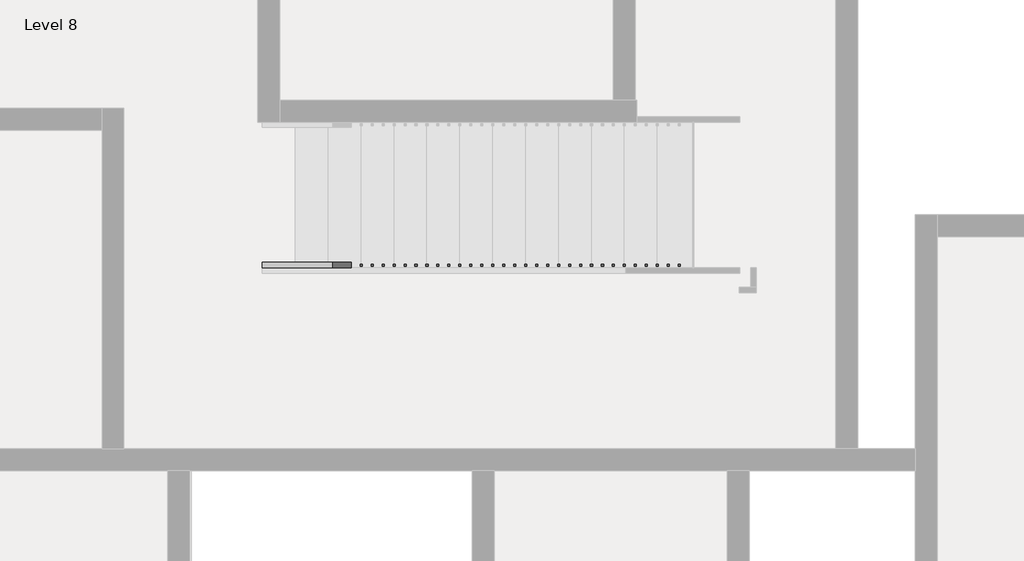
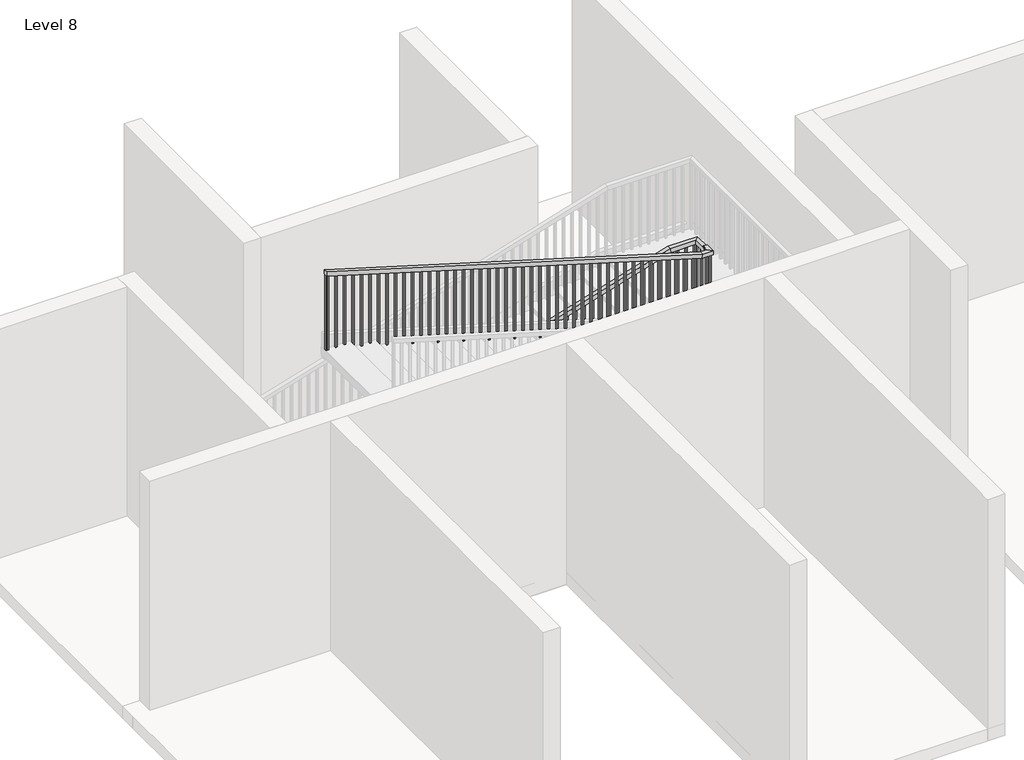
# One storey, part 11 of 14: 1 railing.
"""IFC4 building model written with IfcOpenShell, lengths in millimetres."""

from ifc_helpers import new_model, si_unit, frame, origin, place, context, project, spatial, polyline, outline, extrude, faceted_brep, element, save

model = new_model("IFC4")

# Units and contexts
model_context = context("Model", 3, world=origin())
ifc_project = project(units=[si_unit("LENGTHUNIT", "METRE", prefix="MILLI")], contexts=[model_context])

# Site, building, storey
site = spatial("IfcSite", under=ifc_project)
building = spatial("IfcBuilding", under=site)
storey = spatial("IfcBuildingStorey", under=building, Name="Level 8", Elevation=21336.0)

# Railing
placement = place(None, origin())
element("IfcRailing", 1, ObjectType="Handrail - Rectangular", at=placement, inside=storey, context=model_context, shape_type="SolidModel", body=[
    faceted_brep([(-5254.0891351, 11205.0082924, 22341.84), (-5254.0891351, 11205.0082924, 22288.8032429), (-5254.0891351, 11154.2082924, 22288.8032429), (-5254.0891351, 11154.2082924, 22341.84), (-986.8891351, 11205.0082924, 23622.0), (-979.4332782, 11205.0082924, 23571.2), (-979.4332782, 11154.2082924, 23571.2), (-986.8891351, 11154.2082924, 23622.0), (-631.2891351, 11205.0082924, 23622.0), (-631.2891351, 11205.0082924, 23571.2), (-682.0891351, 11154.2082924, 23571.2), (-682.0891351, 11154.2082924, 23622.0), (-631.2891351, 11001.8082924, 23622.0), (-631.2891351, 10951.0082924, 23571.2), (-682.0891351, 10951.0082924, 23571.2), (-682.0891351, 11001.8082924, 23622.0), (-631.2891351, 11001.8082924, 23644.86), (-631.2891351, 10951.0082924, 23594.06), (-682.0891351, 10951.0082924, 23594.06), (-682.0891351, 11001.8082924, 23644.86), (-631.2891351, 10874.8082924, 23644.86), (-631.2891351, 10874.8082924, 23594.06), (-682.0891351, 10925.6082924, 23594.06), (-682.0891351, 10925.6082924, 23644.86), (-758.2891351, 10874.8082924, 23644.86), (-765.744992, 10874.8082924, 23594.06), (-765.744992, 10925.6082924, 23594.06), (-758.2891351, 10925.6082924, 23644.86), (-5254.0891351, 10874.8082924, 24993.6), (-5254.0891351, 10925.6082924, 24993.6), (-5254.0891351, 10925.6082924, 24940.5632429), (-5254.0891351, 10874.8082924, 24940.5632429)], [[[0, 1, 2, 3]], [[1, 0, 4, 5]], [[2, 1, 5, 6]], [[3, 2, 6, 7]], [[0, 3, 7, 4]], [[5, 4, 8, 9]], [[6, 5, 9, 10]], [[7, 6, 10, 11]], [[4, 7, 11, 8]], [[9, 8, 12, 13]], [[10, 9, 13, 14]], [[11, 10, 14, 15]], [[8, 11, 15, 12]], [[13, 12, 16, 17]], [[14, 13, 17, 18]], [[15, 14, 18, 19]], [[12, 15, 19, 16]], [[17, 16, 20, 21]], [[18, 17, 21, 22]], [[19, 18, 22, 23]], [[16, 19, 23, 20]], [[21, 20, 24, 25]], [[22, 21, 25, 26]], [[23, 22, 26, 27]], [[20, 23, 27, 24]], [[28, 29, 30, 31]], [[25, 24, 28, 31]], [[26, 25, 31, 30]], [[27, 26, 30, 29]], [[24, 27, 29, 28]]]),
    extrude(outline(polyline([(24930.0857429, -5219.1641351), (24935.8007429, -5238.2141351), (23987.76, -5238.2141351), (23987.76, -5219.1641351), (24930.0857429, -5219.1641351)])), frame((0.0, 10890.6832924, 0.0), z_axis=(0.0, 1.0, 0.0), x_axis=(0.0, 0.0, 1.0)), (0.0, 0.0, 1.0), 19.05),
    extrude(outline(polyline([(24899.6057429, -5117.5641351), (24905.3207429, -5136.6141351), (23987.76, -5136.6141351), (23987.76, -5117.5641351), (24899.6057429, -5117.5641351)])), frame((0.0, 10890.6832924, 0.0), z_axis=(0.0, 1.0, 0.0), x_axis=(0.0, 0.0, 1.0)), (0.0, 0.0, 1.0), 19.05),
    extrude(outline(polyline([(24869.1257429, -5015.9641351), (24874.8407429, -5035.0141351), (23987.76, -5035.0141351), (23987.76, -5015.9641351), (24869.1257429, -5015.9641351)])), frame((0.0, 10890.6832924, 0.0), z_axis=(0.0, 1.0, 0.0), x_axis=(0.0, 0.0, 1.0)), (0.0, 0.0, 1.0), 19.05),
    extrude(outline(polyline([(24838.6457429, -4914.3641351), (24844.3607429, -4933.4141351), (23896.32, -4933.4141351), (23896.32, -4914.3641351), (24838.6457429, -4914.3641351)])), frame((0.0, 10890.6832924, 0.0), z_axis=(0.0, 1.0, 0.0), x_axis=(0.0, 0.0, 1.0)), (0.0, 0.0, 1.0), 19.05),
    extrude(outline(polyline([(24808.1657429, -4812.7641351), (24813.8807429, -4831.8141351), (23896.32, -4831.8141351), (23896.32, -4812.7641351), (24808.1657429, -4812.7641351)])), frame((0.0, 10890.6832924, 0.0), z_axis=(0.0, 1.0, 0.0), x_axis=(0.0, 0.0, 1.0)), (0.0, 0.0, 1.0), 19.05),
    extrude(outline(polyline([(24777.6857429, -4711.1641351), (24783.4007429, -4730.2141351), (23896.32, -4730.2141351), (23896.32, -4711.1641351), (24777.6857429, -4711.1641351)])), frame((0.0, 10890.6832924, 0.0), z_axis=(0.0, 1.0, 0.0), x_axis=(0.0, 0.0, 1.0)), (0.0, 0.0, 1.0), 19.05),
    extrude(outline(polyline([(24747.2057429, -4609.5641351), (24752.9207429, -4628.6141351), (23804.88, -4628.6141351), (23804.88, -4609.5641351), (24747.2057429, -4609.5641351)])), frame((0.0, 10890.6832924, 0.0), z_axis=(0.0, 1.0, 0.0), x_axis=(0.0, 0.0, 1.0)), (0.0, 0.0, 1.0), 19.05),
    extrude(outline(polyline([(24716.7257429, -4507.9641351), (24722.4407429, -4527.0141351), (23804.88, -4527.0141351), (23804.88, -4507.9641351), (24716.7257429, -4507.9641351)])), frame((0.0, 10890.6832924, 0.0), z_axis=(0.0, 1.0, 0.0), x_axis=(0.0, 0.0, 1.0)), (0.0, 0.0, 1.0), 19.05),
    extrude(outline(polyline([(24686.2457429, -4406.3641351), (24691.9607429, -4425.4141351), (23804.88, -4425.4141351), (23804.88, -4406.3641351), (24686.2457429, -4406.3641351)])), frame((0.0, 10890.6832924, 0.0), z_axis=(0.0, 1.0, 0.0), x_axis=(0.0, 0.0, 1.0)), (0.0, 0.0, 1.0), 19.05),
    extrude(outline(polyline([(24655.7657429, -4304.7641351), (24661.4807429, -4323.8141351), (23713.44, -4323.8141351), (23713.44, -4304.7641351), (24655.7657429, -4304.7641351)])), frame((0.0, 10890.6832924, 0.0), z_axis=(0.0, 1.0, 0.0), x_axis=(0.0, 0.0, 1.0)), (0.0, 0.0, 1.0), 19.05),
    extrude(outline(polyline([(24625.2857429, -4203.1641351), (24631.0007429, -4222.2141351), (23713.44, -4222.2141351), (23713.44, -4203.1641351), (24625.2857429, -4203.1641351)])), frame((0.0, 10890.6832924, 0.0), z_axis=(0.0, 1.0, 0.0), x_axis=(0.0, 0.0, 1.0)), (0.0, 0.0, 1.0), 19.05),
    extrude(outline(polyline([(24594.8057429, -4101.5641351), (24600.5207429, -4120.6141351), (23713.44, -4120.6141351), (23713.44, -4101.5641351), (24594.8057429, -4101.5641351)])), frame((0.0, 10890.6832924, 0.0), z_axis=(0.0, 1.0, 0.0), x_axis=(0.0, 0.0, 1.0)), (0.0, 0.0, 1.0), 19.05),
    extrude(outline(polyline([(24564.3257429, -3999.9641351), (24570.0407429, -4019.0141351), (23622.0, -4019.0141351), (23622.0, -3999.9641351), (24564.3257429, -3999.9641351)])), frame((0.0, 10890.6832924, 0.0), z_axis=(0.0, 1.0, 0.0), x_axis=(0.0, 0.0, 1.0)), (0.0, 0.0, 1.0), 19.05),
    extrude(outline(polyline([(24533.8457429, -3898.3641351), (24539.5607429, -3917.4141351), (23622.0, -3917.4141351), (23622.0, -3898.3641351), (24533.8457429, -3898.3641351)])), frame((0.0, 10890.6832924, 0.0), z_axis=(0.0, 1.0, 0.0), x_axis=(0.0, 0.0, 1.0)), (0.0, 0.0, 1.0), 19.05),
    extrude(outline(polyline([(24503.3657429, -3796.7641351), (24509.0807429, -3815.8141351), (23622.0, -3815.8141351), (23622.0, -3796.7641351), (24503.3657429, -3796.7641351)])), frame((0.0, 10890.6832924, 0.0), z_axis=(0.0, 1.0, 0.0), x_axis=(0.0, 0.0, 1.0)), (0.0, 0.0, 1.0), 19.05),
    extrude(outline(polyline([(24472.8857429, -3695.1641351), (24478.6007429, -3714.2141351), (23530.56, -3714.2141351), (23530.56, -3695.1641351), (24472.8857429, -3695.1641351)])), frame((0.0, 10890.6832924, 0.0), z_axis=(0.0, 1.0, 0.0), x_axis=(0.0, 0.0, 1.0)), (0.0, 0.0, 1.0), 19.05),
    extrude(outline(polyline([(24442.4057429, -3593.5641351), (24448.1207429, -3612.6141351), (23530.56, -3612.6141351), (23530.56, -3593.5641351), (24442.4057429, -3593.5641351)])), frame((0.0, 10890.6832924, 0.0), z_axis=(0.0, 1.0, 0.0), x_axis=(0.0, 0.0, 1.0)), (0.0, 0.0, 1.0), 19.05),
    extrude(outline(polyline([(24411.9257429, -3491.9641351), (24417.6407429, -3511.0141351), (23530.56, -3511.0141351), (23530.56, -3491.9641351), (24411.9257429, -3491.9641351)])), frame((0.0, 10890.6832924, 0.0), z_axis=(0.0, 1.0, 0.0), x_axis=(0.0, 0.0, 1.0)), (0.0, 0.0, 1.0), 19.05),
    extrude(outline(polyline([(24381.4457429, -3390.3641351), (24387.1607429, -3409.4141351), (23439.12, -3409.4141351), (23439.12, -3390.3641351), (24381.4457429, -3390.3641351)])), frame((0.0, 10890.6832924, 0.0), z_axis=(0.0, 1.0, 0.0), x_axis=(0.0, 0.0, 1.0)), (0.0, 0.0, 1.0), 19.05),
    extrude(outline(polyline([(24350.9657429, -3288.7641351), (24356.6807429, -3307.8141351), (23439.12, -3307.8141351), (23439.12, -3288.7641351), (24350.9657429, -3288.7641351)])), frame((0.0, 10890.6832924, 0.0), z_axis=(0.0, 1.0, 0.0), x_axis=(0.0, 0.0, 1.0)), (0.0, 0.0, 1.0), 19.05),
    extrude(outline(polyline([(24320.4857429, -3187.1641351), (24326.2007429, -3206.2141351), (23439.12, -3206.2141351), (23439.12, -3187.1641351), (24320.4857429, -3187.1641351)])), frame((0.0, 10890.6832924, 0.0), z_axis=(0.0, 1.0, 0.0), x_axis=(0.0, 0.0, 1.0)), (0.0, 0.0, 1.0), 19.05),
    extrude(outline(polyline([(24290.0057429, -3085.5641351), (24295.7207429, -3104.6141351), (23347.68, -3104.6141351), (23347.68, -3085.5641351), (24290.0057429, -3085.5641351)])), frame((0.0, 10890.6832924, 0.0), z_axis=(0.0, 1.0, 0.0), x_axis=(0.0, 0.0, 1.0)), (0.0, 0.0, 1.0), 19.05),
    extrude(outline(polyline([(24259.5257429, -2983.9641351), (24265.2407429, -3003.0141351), (23347.68, -3003.0141351), (23347.68, -2983.9641351), (24259.5257429, -2983.9641351)])), frame((0.0, 10890.6832924, 0.0), z_axis=(0.0, 1.0, 0.0), x_axis=(0.0, 0.0, 1.0)), (0.0, 0.0, 1.0), 19.05),
    extrude(outline(polyline([(24229.0457429, -2882.3641351), (24234.7607429, -2901.4141351), (23347.68, -2901.4141351), (23347.68, -2882.3641351), (24229.0457429, -2882.3641351)])), frame((0.0, 10890.6832924, 0.0), z_axis=(0.0, 1.0, 0.0), x_axis=(0.0, 0.0, 1.0)), (0.0, 0.0, 1.0), 19.05),
    extrude(outline(polyline([(24198.5657429, -2780.7641351), (24204.2807429, -2799.8141351), (23256.24, -2799.8141351), (23256.24, -2780.7641351), (24198.5657429, -2780.7641351)])), frame((0.0, 10890.6832924, 0.0), z_axis=(0.0, 1.0, 0.0), x_axis=(0.0, 0.0, 1.0)), (0.0, 0.0, 1.0), 19.05),
    extrude(outline(polyline([(24168.0857429, -2679.1641351), (24173.8007429, -2698.2141351), (23256.24, -2698.2141351), (23256.24, -2679.1641351), (24168.0857429, -2679.1641351)])), frame((0.0, 10890.6832924, 0.0), z_axis=(0.0, 1.0, 0.0), x_axis=(0.0, 0.0, 1.0)), (0.0, 0.0, 1.0), 19.05),
    extrude(outline(polyline([(24137.6057429, -2577.5641351), (24143.3207429, -2596.6141351), (23256.24, -2596.6141351), (23256.24, -2577.5641351), (24137.6057429, -2577.5641351)])), frame((0.0, 10890.6832924, 0.0), z_axis=(0.0, 1.0, 0.0), x_axis=(0.0, 0.0, 1.0)), (0.0, 0.0, 1.0), 19.05),
    extrude(outline(polyline([(24107.1257429, -2475.9641351), (24112.8407429, -2495.0141351), (23164.8, -2495.0141351), (23164.8, -2475.9641351), (24107.1257429, -2475.9641351)])), frame((0.0, 10890.6832924, 0.0), z_axis=(0.0, 1.0, 0.0), x_axis=(0.0, 0.0, 1.0)), (0.0, 0.0, 1.0), 19.05),
    extrude(outline(polyline([(24076.6457429, -2374.3641351), (24082.3607429, -2393.4141351), (23164.8, -2393.4141351), (23164.8, -2374.3641351), (24076.6457429, -2374.3641351)])), frame((0.0, 10890.6832924, 0.0), z_axis=(0.0, 1.0, 0.0), x_axis=(0.0, 0.0, 1.0)), (0.0, 0.0, 1.0), 19.05),
    extrude(outline(polyline([(24046.1657429, -2272.7641351), (24051.8807429, -2291.8141351), (23164.8, -2291.8141351), (23164.8, -2272.7641351), (24046.1657429, -2272.7641351)])), frame((0.0, 10890.6832924, 0.0), z_axis=(0.0, 1.0, 0.0), x_axis=(0.0, 0.0, 1.0)), (0.0, 0.0, 1.0), 19.05),
    extrude(outline(polyline([(24015.6857429, -2171.1641351), (24021.4007429, -2190.2141351), (23073.36, -2190.2141351), (23073.36, -2171.1641351), (24015.6857429, -2171.1641351)])), frame((0.0, 10890.6832924, 0.0), z_axis=(0.0, 1.0, 0.0), x_axis=(0.0, 0.0, 1.0)), (0.0, 0.0, 1.0), 19.05),
    extrude(outline(polyline([(23985.2057429, -2069.5641351), (23990.9207429, -2088.6141351), (23073.36, -2088.6141351), (23073.36, -2069.5641351), (23985.2057429, -2069.5641351)])), frame((0.0, 10890.6832924, 0.0), z_axis=(0.0, 1.0, 0.0), x_axis=(0.0, 0.0, 1.0)), (0.0, 0.0, 1.0), 19.05),
    extrude(outline(polyline([(23954.7257429, -1967.9641351), (23960.4407429, -1987.0141351), (23073.36, -1987.0141351), (23073.36, -1967.9641351), (23954.7257429, -1967.9641351)])), frame((0.0, 10890.6832924, 0.0), z_axis=(0.0, 1.0, 0.0), x_axis=(0.0, 0.0, 1.0)), (0.0, 0.0, 1.0), 19.05),
    extrude(outline(polyline([(23924.2457429, -1866.3641351), (23929.9607429, -1885.4141351), (22981.92, -1885.4141351), (22981.92, -1866.3641351), (23924.2457429, -1866.3641351)])), frame((0.0, 10890.6832924, 0.0), z_axis=(0.0, 1.0, 0.0), x_axis=(0.0, 0.0, 1.0)), (0.0, 0.0, 1.0), 19.05),
    extrude(outline(polyline([(23893.7657429, -1764.7641351), (23899.4807429, -1783.8141351), (22981.92, -1783.8141351), (22981.92, -1764.7641351), (23893.7657429, -1764.7641351)])), frame((0.0, 10890.6832924, 0.0), z_axis=(0.0, 1.0, 0.0), x_axis=(0.0, 0.0, 1.0)), (0.0, 0.0, 1.0), 19.05),
    extrude(outline(polyline([(23863.2857429, -1663.1641351), (23869.0007429, -1682.2141351), (22981.92, -1682.2141351), (22981.92, -1663.1641351), (23863.2857429, -1663.1641351)])), frame((0.0, 10890.6832924, 0.0), z_axis=(0.0, 1.0, 0.0), x_axis=(0.0, 0.0, 1.0)), (0.0, 0.0, 1.0), 19.05),
    extrude(outline(polyline([(23832.8057429, -1561.5641351), (23838.5207429, -1580.6141351), (22890.48, -1580.6141351), (22890.48, -1561.5641351), (23832.8057429, -1561.5641351)])), frame((0.0, 10890.6832924, 0.0), z_axis=(0.0, 1.0, 0.0), x_axis=(0.0, 0.0, 1.0)), (0.0, 0.0, 1.0), 19.05),
    extrude(outline(polyline([(23802.3257429, -1459.9641351), (23808.0407429, -1479.0141351), (22890.48, -1479.0141351), (22890.48, -1459.9641351), (23802.3257429, -1459.9641351)])), frame((0.0, 10890.6832924, 0.0), z_axis=(0.0, 1.0, 0.0), x_axis=(0.0, 0.0, 1.0)), (0.0, 0.0, 1.0), 19.05),
    extrude(outline(polyline([(23771.8457429, -1358.3641351), (23777.5607429, -1377.4141351), (22890.48, -1377.4141351), (22890.48, -1358.3641351), (23771.8457429, -1358.3641351)])), frame((0.0, 10890.6832924, 0.0), z_axis=(0.0, 1.0, 0.0), x_axis=(0.0, 0.0, 1.0)), (0.0, 0.0, 1.0), 19.05),
    extrude(outline(polyline([(23741.3657429, -1256.7641351), (23747.0807429, -1275.8141351), (22799.04, -1275.8141351), (22799.04, -1256.7641351), (23741.3657429, -1256.7641351)])), frame((0.0, 10890.6832924, 0.0), z_axis=(0.0, 1.0, 0.0), x_axis=(0.0, 0.0, 1.0)), (0.0, 0.0, 1.0), 19.05),
    extrude(outline(polyline([(23710.8857429, -1155.1641351), (23716.6007429, -1174.2141351), (22799.04, -1174.2141351), (22799.04, -1155.1641351), (23710.8857429, -1155.1641351)])), frame((0.0, 10890.6832924, 0.0), z_axis=(0.0, 1.0, 0.0), x_axis=(0.0, 0.0, 1.0)), (0.0, 0.0, 1.0), 19.05),
    extrude(outline(polyline([(23680.4057429, -1053.5641351), (23686.1207429, -1072.6141351), (22799.04, -1072.6141351), (22799.04, -1053.5641351), (23680.4057429, -1053.5641351)])), frame((0.0, 10890.6832924, 0.0), z_axis=(0.0, 1.0, 0.0), x_axis=(0.0, 0.0, 1.0)), (0.0, 0.0, 1.0), 19.05),
    extrude(outline(polyline([(23649.9257429, -951.9641351), (23655.6407429, -971.0141351), (22707.6, -971.0141351), (22707.6, -951.9641351), (23649.9257429, -951.9641351)])), frame((0.0, 10890.6832924, 0.0), z_axis=(0.0, 1.0, 0.0), x_axis=(0.0, 0.0, 1.0)), (0.0, 0.0, 1.0), 19.05),
    extrude(outline(polyline([(23619.4457429, -850.3641351), (23625.1607429, -869.4141351), (22707.6, -869.4141351), (22707.6, -850.3641351), (23619.4457429, -850.3641351)])), frame((0.0, 10890.6832924, 0.0), z_axis=(0.0, 1.0, 0.0), x_axis=(0.0, 0.0, 1.0)), (0.0, 0.0, 1.0), 19.05),
    extrude(outline(polyline([(23588.9657429, -748.7641351), (23594.6807429, -767.8141351), (22707.6, -767.8141351), (22707.6, -748.7641351), (23588.9657429, -748.7641351)])), frame((0.0, 10890.6832924, 0.0), z_axis=(0.0, 1.0, 0.0), x_axis=(0.0, 0.0, 1.0)), (0.0, 0.0, 1.0), 19.05),
    extrude(outline(polyline([(-666.2141351, 10985.9332924), (-647.1641351, 10985.9332924), (-647.1641351, 10966.8832924), (-666.2141351, 10966.8832924), (-666.2141351, 10985.9332924)])), frame((0.0, 0.0, 22707.6), z_axis=(0.0, 0.0, 1.0), x_axis=(1.0, 0.0, 0.0)), (0.0, 0.0, 1.0), 886.46),
    extrude(outline(polyline([(-666.2141351, 11087.5332924), (-647.1641351, 11087.5332924), (-647.1641351, 11068.4832924), (-666.2141351, 11068.4832924), (-666.2141351, 11087.5332924)])), frame((0.0, 0.0, 22707.6), z_axis=(0.0, 0.0, 1.0), x_axis=(1.0, 0.0, 0.0)), (0.0, 0.0, 1.0), 863.6),
    extrude(outline(polyline([(-691.6141351, 11170.0832924), (-691.6141351, 11189.1332924), (-672.5641351, 11189.1332924), (-672.5641351, 11170.0832924), (-691.6141351, 11170.0832924)])), frame((0.0, 0.0, 22707.6), z_axis=(0.0, 0.0, 1.0), x_axis=(1.0, 0.0, 0.0)), (0.0, 0.0, 1.0), 863.6),
    extrude(outline(polyline([(-793.2141351, 11170.0832924), (-793.2141351, 11189.1332924), (-774.1641351, 11189.1332924), (-774.1641351, 11170.0832924), (-793.2141351, 11170.0832924)])), frame((0.0, 0.0, 22707.6), z_axis=(0.0, 0.0, 1.0), x_axis=(1.0, 0.0, 0.0)), (0.0, 0.0, 1.0), 863.6),
    extrude(outline(polyline([(-894.8141351, 11170.0832924), (-894.8141351, 11189.1332924), (-875.7641351, 11189.1332924), (-875.7641351, 11170.0832924), (-894.8141351, 11170.0832924)])), frame((0.0, 0.0, 22707.6), z_axis=(0.0, 0.0, 1.0), x_axis=(1.0, 0.0, 0.0)), (0.0, 0.0, 1.0), 863.6),
    extrude(outline(polyline([(23571.8207429, -977.3641351), (23566.1057429, -996.4141351), (22707.6, -996.4141351), (22707.6, -977.3641351), (23571.8207429, -977.3641351)])), frame((0.0, 11170.0832924, 0.0), z_axis=(0.0, 1.0, 0.0), x_axis=(0.0, 0.0, 1.0)), (0.0, 0.0, 1.0), 19.05),
    extrude(outline(polyline([(23541.3407429, -1078.9641351), (23535.6257429, -1098.0141351), (22616.16, -1098.0141351), (22616.16, -1078.9641351), (23541.3407429, -1078.9641351)])), frame((0.0, 11170.0832924, 0.0), z_axis=(0.0, 1.0, 0.0), x_axis=(0.0, 0.0, 1.0)), (0.0, 0.0, 1.0), 19.05),
    extrude(outline(polyline([(23510.8607429, -1180.5641351), (23505.1457429, -1199.6141351), (22616.16, -1199.6141351), (22616.16, -1180.5641351), (23510.8607429, -1180.5641351)])), frame((0.0, 11170.0832924, 0.0), z_axis=(0.0, 1.0, 0.0), x_axis=(0.0, 0.0, 1.0)), (0.0, 0.0, 1.0), 19.05),
    extrude(outline(polyline([(23480.3807429, -1282.1641351), (23474.6657429, -1301.2141351), (22616.16, -1301.2141351), (22616.16, -1282.1641351), (23480.3807429, -1282.1641351)])), frame((0.0, 11170.0832924, 0.0), z_axis=(0.0, 1.0, 0.0), x_axis=(0.0, 0.0, 1.0)), (0.0, 0.0, 1.0), 19.05),
    extrude(outline(polyline([(23449.9007429, -1383.7641351), (23444.1857429, -1402.8141351), (22524.72, -1402.8141351), (22524.72, -1383.7641351), (23449.9007429, -1383.7641351)])), frame((0.0, 11170.0832924, 0.0), z_axis=(0.0, 1.0, 0.0), x_axis=(0.0, 0.0, 1.0)), (0.0, 0.0, 1.0), 19.05),
    extrude(outline(polyline([(23419.4207429, -1485.3641351), (23413.7057429, -1504.4141351), (22524.72, -1504.4141351), (22524.72, -1485.3641351), (23419.4207429, -1485.3641351)])), frame((0.0, 11170.0832924, 0.0), z_axis=(0.0, 1.0, 0.0), x_axis=(0.0, 0.0, 1.0)), (0.0, 0.0, 1.0), 19.05),
    extrude(outline(polyline([(23388.9407429, -1586.9641351), (23383.2257429, -1606.0141351), (22524.72, -1606.0141351), (22524.72, -1586.9641351), (23388.9407429, -1586.9641351)])), frame((0.0, 11170.0832924, 0.0), z_axis=(0.0, 1.0, 0.0), x_axis=(0.0, 0.0, 1.0)), (0.0, 0.0, 1.0), 19.05),
    extrude(outline(polyline([(23358.4607429, -1688.5641351), (23352.7457429, -1707.6141351), (22433.28, -1707.6141351), (22433.28, -1688.5641351), (23358.4607429, -1688.5641351)])), frame((0.0, 11170.0832924, 0.0), z_axis=(0.0, 1.0, 0.0), x_axis=(0.0, 0.0, 1.0)), (0.0, 0.0, 1.0), 19.05),
    extrude(outline(polyline([(23327.9807429, -1790.1641351), (23322.2657429, -1809.2141351), (22433.28, -1809.2141351), (22433.28, -1790.1641351), (23327.9807429, -1790.1641351)])), frame((0.0, 11170.0832924, 0.0), z_axis=(0.0, 1.0, 0.0), x_axis=(0.0, 0.0, 1.0)), (0.0, 0.0, 1.0), 19.05),
    extrude(outline(polyline([(23297.5007429, -1891.7641351), (23291.7857429, -1910.8141351), (22433.28, -1910.8141351), (22433.28, -1891.7641351), (23297.5007429, -1891.7641351)])), frame((0.0, 11170.0832924, 0.0), z_axis=(0.0, 1.0, 0.0), x_axis=(0.0, 0.0, 1.0)), (0.0, 0.0, 1.0), 19.05),
    extrude(outline(polyline([(23267.0207429, -1993.3641351), (23261.3057429, -2012.4141351), (22341.84, -2012.4141351), (22341.84, -1993.3641351), (23267.0207429, -1993.3641351)])), frame((0.0, 11170.0832924, 0.0), z_axis=(0.0, 1.0, 0.0), x_axis=(0.0, 0.0, 1.0)), (0.0, 0.0, 1.0), 19.05),
    extrude(outline(polyline([(23236.5407429, -2094.9641351), (23230.8257429, -2114.0141351), (22341.84, -2114.0141351), (22341.84, -2094.9641351), (23236.5407429, -2094.9641351)])), frame((0.0, 11170.0832924, 0.0), z_axis=(0.0, 1.0, 0.0), x_axis=(0.0, 0.0, 1.0)), (0.0, 0.0, 1.0), 19.05),
    extrude(outline(polyline([(23206.0607429, -2196.5641351), (23200.3457429, -2215.6141351), (22341.84, -2215.6141351), (22341.84, -2196.5641351), (23206.0607429, -2196.5641351)])), frame((0.0, 11170.0832924, 0.0), z_axis=(0.0, 1.0, 0.0), x_axis=(0.0, 0.0, 1.0)), (0.0, 0.0, 1.0), 19.05),
    extrude(outline(polyline([(23175.5807429, -2298.1641351), (23169.8657429, -2317.2141351), (22250.4, -2317.2141351), (22250.4, -2298.1641351), (23175.5807429, -2298.1641351)])), frame((0.0, 11170.0832924, 0.0), z_axis=(0.0, 1.0, 0.0), x_axis=(0.0, 0.0, 1.0)), (0.0, 0.0, 1.0), 19.05),
    extrude(outline(polyline([(23145.1007429, -2399.7641351), (23139.3857429, -2418.8141351), (22250.4, -2418.8141351), (22250.4, -2399.7641351), (23145.1007429, -2399.7641351)])), frame((0.0, 11170.0832924, 0.0), z_axis=(0.0, 1.0, 0.0), x_axis=(0.0, 0.0, 1.0)), (0.0, 0.0, 1.0), 19.05),
    extrude(outline(polyline([(23114.6207429, -2501.3641351), (23108.9057429, -2520.4141351), (22250.4, -2520.4141351), (22250.4, -2501.3641351), (23114.6207429, -2501.3641351)])), frame((0.0, 11170.0832924, 0.0), z_axis=(0.0, 1.0, 0.0), x_axis=(0.0, 0.0, 1.0)), (0.0, 0.0, 1.0), 19.05),
    extrude(outline(polyline([(23084.1407429, -2602.9641351), (23078.4257429, -2622.0141351), (22158.96, -2622.0141351), (22158.96, -2602.9641351), (23084.1407429, -2602.9641351)])), frame((0.0, 11170.0832924, 0.0), z_axis=(0.0, 1.0, 0.0), x_axis=(0.0, 0.0, 1.0)), (0.0, 0.0, 1.0), 19.05),
    extrude(outline(polyline([(23053.6607429, -2704.5641351), (23047.9457429, -2723.6141351), (22158.96, -2723.6141351), (22158.96, -2704.5641351), (23053.6607429, -2704.5641351)])), frame((0.0, 11170.0832924, 0.0), z_axis=(0.0, 1.0, 0.0), x_axis=(0.0, 0.0, 1.0)), (0.0, 0.0, 1.0), 19.05),
    extrude(outline(polyline([(23023.1807429, -2806.1641351), (23017.4657429, -2825.2141351), (22158.96, -2825.2141351), (22158.96, -2806.1641351), (23023.1807429, -2806.1641351)])), frame((0.0, 11170.0832924, 0.0), z_axis=(0.0, 1.0, 0.0), x_axis=(0.0, 0.0, 1.0)), (0.0, 0.0, 1.0), 19.05),
    extrude(outline(polyline([(22992.7007429, -2907.7641351), (22986.9857429, -2926.8141351), (22067.52, -2926.8141351), (22067.52, -2907.7641351), (22992.7007429, -2907.7641351)])), frame((0.0, 11170.0832924, 0.0), z_axis=(0.0, 1.0, 0.0), x_axis=(0.0, 0.0, 1.0)), (0.0, 0.0, 1.0), 19.05),
    extrude(outline(polyline([(22962.2207429, -3009.3641351), (22956.5057429, -3028.4141351), (22067.52, -3028.4141351), (22067.52, -3009.3641351), (22962.2207429, -3009.3641351)])), frame((0.0, 11170.0832924, 0.0), z_axis=(0.0, 1.0, 0.0), x_axis=(0.0, 0.0, 1.0)), (0.0, 0.0, 1.0), 19.05),
    extrude(outline(polyline([(22931.7407429, -3110.9641351), (22926.0257429, -3130.0141351), (22067.52, -3130.0141351), (22067.52, -3110.9641351), (22931.7407429, -3110.9641351)])), frame((0.0, 11170.0832924, 0.0), z_axis=(0.0, 1.0, 0.0), x_axis=(0.0, 0.0, 1.0)), (0.0, 0.0, 1.0), 19.05),
    extrude(outline(polyline([(22901.2607429, -3212.5641351), (22895.5457429, -3231.6141351), (21976.08, -3231.6141351), (21976.08, -3212.5641351), (22901.2607429, -3212.5641351)])), frame((0.0, 11170.0832924, 0.0), z_axis=(0.0, 1.0, 0.0), x_axis=(0.0, 0.0, 1.0)), (0.0, 0.0, 1.0), 19.05),
    extrude(outline(polyline([(22870.7807429, -3314.1641351), (22865.0657429, -3333.2141351), (21976.08, -3333.2141351), (21976.08, -3314.1641351), (22870.7807429, -3314.1641351)])), frame((0.0, 11170.0832924, 0.0), z_axis=(0.0, 1.0, 0.0), x_axis=(0.0, 0.0, 1.0)), (0.0, 0.0, 1.0), 19.05),
    extrude(outline(polyline([(22840.3007429, -3415.7641351), (22834.5857429, -3434.8141351), (21976.08, -3434.8141351), (21976.08, -3415.7641351), (22840.3007429, -3415.7641351)])), frame((0.0, 11170.0832924, 0.0), z_axis=(0.0, 1.0, 0.0), x_axis=(0.0, 0.0, 1.0)), (0.0, 0.0, 1.0), 19.05),
    extrude(outline(polyline([(22809.8207429, -3517.3641351), (22804.1057429, -3536.4141351), (21884.64, -3536.4141351), (21884.64, -3517.3641351), (22809.8207429, -3517.3641351)])), frame((0.0, 11170.0832924, 0.0), z_axis=(0.0, 1.0, 0.0), x_axis=(0.0, 0.0, 1.0)), (0.0, 0.0, 1.0), 19.05),
    extrude(outline(polyline([(22779.3407429, -3618.9641351), (22773.6257429, -3638.0141351), (21884.64, -3638.0141351), (21884.64, -3618.9641351), (22779.3407429, -3618.9641351)])), frame((0.0, 11170.0832924, 0.0), z_axis=(0.0, 1.0, 0.0), x_axis=(0.0, 0.0, 1.0)), (0.0, 0.0, 1.0), 19.05),
    extrude(outline(polyline([(22748.8607429, -3720.5641351), (22743.1457429, -3739.6141351), (21884.64, -3739.6141351), (21884.64, -3720.5641351), (22748.8607429, -3720.5641351)])), frame((0.0, 11170.0832924, 0.0), z_axis=(0.0, 1.0, 0.0), x_axis=(0.0, 0.0, 1.0)), (0.0, 0.0, 1.0), 19.05),
    extrude(outline(polyline([(22718.3807429, -3822.1641351), (22712.6657429, -3841.2141351), (21793.2, -3841.2141351), (21793.2, -3822.1641351), (22718.3807429, -3822.1641351)])), frame((0.0, 11170.0832924, 0.0), z_axis=(0.0, 1.0, 0.0), x_axis=(0.0, 0.0, 1.0)), (0.0, 0.0, 1.0), 19.05),
    extrude(outline(polyline([(22687.9007429, -3923.7641351), (22682.1857429, -3942.8141351), (21793.2, -3942.8141351), (21793.2, -3923.7641351), (22687.9007429, -3923.7641351)])), frame((0.0, 11170.0832924, 0.0), z_axis=(0.0, 1.0, 0.0), x_axis=(0.0, 0.0, 1.0)), (0.0, 0.0, 1.0), 19.05),
    extrude(outline(polyline([(22657.4207429, -4025.3641351), (22651.7057429, -4044.4141351), (21793.2, -4044.4141351), (21793.2, -4025.3641351), (22657.4207429, -4025.3641351)])), frame((0.0, 11170.0832924, 0.0), z_axis=(0.0, 1.0, 0.0), x_axis=(0.0, 0.0, 1.0)), (0.0, 0.0, 1.0), 19.05),
    extrude(outline(polyline([(22626.9407429, -4126.9641351), (22621.2257429, -4146.0141351), (21701.76, -4146.0141351), (21701.76, -4126.9641351), (22626.9407429, -4126.9641351)])), frame((0.0, 11170.0832924, 0.0), z_axis=(0.0, 1.0, 0.0), x_axis=(0.0, 0.0, 1.0)), (0.0, 0.0, 1.0), 19.05),
    extrude(outline(polyline([(22596.4607429, -4228.5641351), (22590.7457429, -4247.6141351), (21701.76, -4247.6141351), (21701.76, -4228.5641351), (22596.4607429, -4228.5641351)])), frame((0.0, 11170.0832924, 0.0), z_axis=(0.0, 1.0, 0.0), x_axis=(0.0, 0.0, 1.0)), (0.0, 0.0, 1.0), 19.05),
    extrude(outline(polyline([(22565.9807429, -4330.1641351), (22560.2657429, -4349.2141351), (21701.76, -4349.2141351), (21701.76, -4330.1641351), (22565.9807429, -4330.1641351)])), frame((0.0, 11170.0832924, 0.0), z_axis=(0.0, 1.0, 0.0), x_axis=(0.0, 0.0, 1.0)), (0.0, 0.0, 1.0), 19.05),
    extrude(outline(polyline([(22535.5007429, -4431.7641351), (22529.7857429, -4450.8141351), (21610.32, -4450.8141351), (21610.32, -4431.7641351), (22535.5007429, -4431.7641351)])), frame((0.0, 11170.0832924, 0.0), z_axis=(0.0, 1.0, 0.0), x_axis=(0.0, 0.0, 1.0)), (0.0, 0.0, 1.0), 19.05),
    extrude(outline(polyline([(22505.0207429, -4533.3641351), (22499.3057429, -4552.4141351), (21610.32, -4552.4141351), (21610.32, -4533.3641351), (22505.0207429, -4533.3641351)])), frame((0.0, 11170.0832924, 0.0), z_axis=(0.0, 1.0, 0.0), x_axis=(0.0, 0.0, 1.0)), (0.0, 0.0, 1.0), 19.05),
    extrude(outline(polyline([(22474.5407429, -4634.9641351), (22468.8257429, -4654.0141351), (21610.32, -4654.0141351), (21610.32, -4634.9641351), (22474.5407429, -4634.9641351)])), frame((0.0, 11170.0832924, 0.0), z_axis=(0.0, 1.0, 0.0), x_axis=(0.0, 0.0, 1.0)), (0.0, 0.0, 1.0), 19.05),
    extrude(outline(polyline([(22444.0607429, -4736.5641351), (22438.3457429, -4755.6141351), (21518.88, -4755.6141351), (21518.88, -4736.5641351), (22444.0607429, -4736.5641351)])), frame((0.0, 11170.0832924, 0.0), z_axis=(0.0, 1.0, 0.0), x_axis=(0.0, 0.0, 1.0)), (0.0, 0.0, 1.0), 19.05),
    extrude(outline(polyline([(22413.5807429, -4838.1641351), (22407.8657429, -4857.2141351), (21518.88, -4857.2141351), (21518.88, -4838.1641351), (22413.5807429, -4838.1641351)])), frame((0.0, 11170.0832924, 0.0), z_axis=(0.0, 1.0, 0.0), x_axis=(0.0, 0.0, 1.0)), (0.0, 0.0, 1.0), 19.05),
    extrude(outline(polyline([(22383.1007429, -4939.7641351), (22377.3857429, -4958.8141351), (21518.88, -4958.8141351), (21518.88, -4939.7641351), (22383.1007429, -4939.7641351)])), frame((0.0, 11170.0832924, 0.0), z_axis=(0.0, 1.0, 0.0), x_axis=(0.0, 0.0, 1.0)), (0.0, 0.0, 1.0), 19.05),
    extrude(outline(polyline([(22352.6207429, -5041.3641351), (22346.9057429, -5060.4141351), (21427.44, -5060.4141351), (21427.44, -5041.3641351), (22352.6207429, -5041.3641351)])), frame((0.0, 11170.0832924, 0.0), z_axis=(0.0, 1.0, 0.0), x_axis=(0.0, 0.0, 1.0)), (0.0, 0.0, 1.0), 19.05),
    extrude(outline(polyline([(22322.1407429, -5142.9641351), (22316.4257429, -5162.0141351), (21427.44, -5162.0141351), (21427.44, -5142.9641351), (22322.1407429, -5142.9641351)])), frame((0.0, 11170.0832924, 0.0), z_axis=(0.0, 1.0, 0.0), x_axis=(0.0, 0.0, 1.0)), (0.0, 0.0, 1.0), 19.05),
    extrude(outline(polyline([(-666.2141351, 10909.7332924), (-647.1641351, 10909.7332924), (-647.1641351, 10890.6832924), (-666.2141351, 10890.6832924), (-666.2141351, 10909.7332924)])), frame((0.0, 0.0, 22707.6), z_axis=(0.0, 0.0, 1.0), x_axis=(1.0, 0.0, 0.0)), (0.0, 0.0, 1.0), 886.46),
    extrude(outline(polyline([(-666.2141351, 11170.0832924), (-666.2141351, 11189.1332924), (-647.1641351, 11189.1332924), (-647.1641351, 11170.0832924), (-666.2141351, 11170.0832924)])), frame((0.0, 0.0, 22707.6), z_axis=(0.0, 0.0, 1.0), x_axis=(1.0, 0.0, 0.0)), (0.0, 0.0, 1.0), 863.6),
    extrude(outline(polyline([(24934.8482429, -5235.0391351), (24940.5632429, -5254.0891351), (23987.76, -5254.0891351), (23987.76, -5235.0391351), (24934.8482429, -5235.0391351)])), frame((0.0, 10890.6832924, 0.0), z_axis=(0.0, 1.0, 0.0), x_axis=(0.0, 0.0, 1.0)), (0.0, 0.0, 1.0), 19.05),
    extrude(outline(polyline([(22294.5182429, -5235.0391351), (22288.8032429, -5254.0891351), (21427.44, -5254.0891351), (21427.44, -5235.0391351), (22294.5182429, -5235.0391351)])), frame((0.0, 11170.0832924, 0.0), z_axis=(0.0, 1.0, 0.0), x_axis=(0.0, 0.0, 1.0)), (0.0, 0.0, 1.0), 19.05),
])

save(model, "model.ifc")

# Revit data of these elements
# Type "Handrail - Rectangular"
#   Assembly Code = "C2010400"
#   built-in parameter 1008612 = 0.0416667 (stored number, unit not read)
#   built-in parameter 1008611 = 0.0416667 (stored number, unit not read)
#   built-in parameter 1008609 = 0.333333 (stored number, unit not read)
#   built-in parameter 1008604 = 0.166667 (stored number, unit not read)
#   built-in parameter 1008603 = 0.166667 (stored number, unit not read)
#   Railing Height = 3' - 0"
#   built-in parameter 1008630 = 2
#   built-in parameter 1008610 = 2
#   built-in parameter 1008618 = Baluster - Square : 3/4"
# Element 1 (IfcRailing, "Handrail - Rectangular")
#   Phase Created = New Construction
